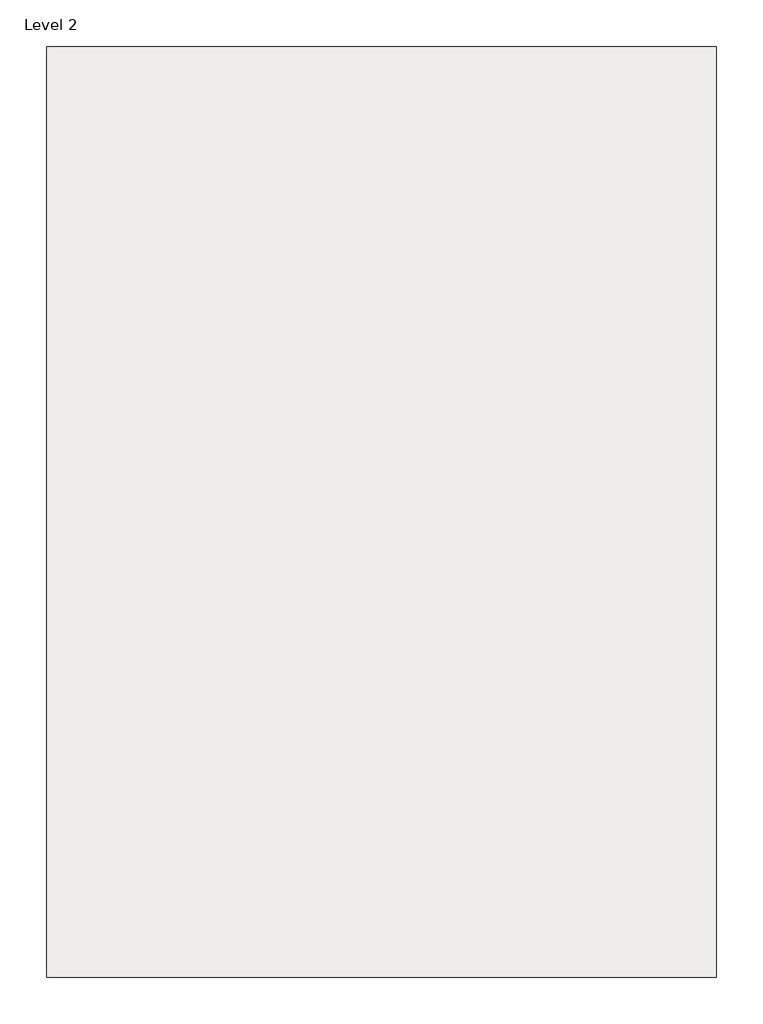
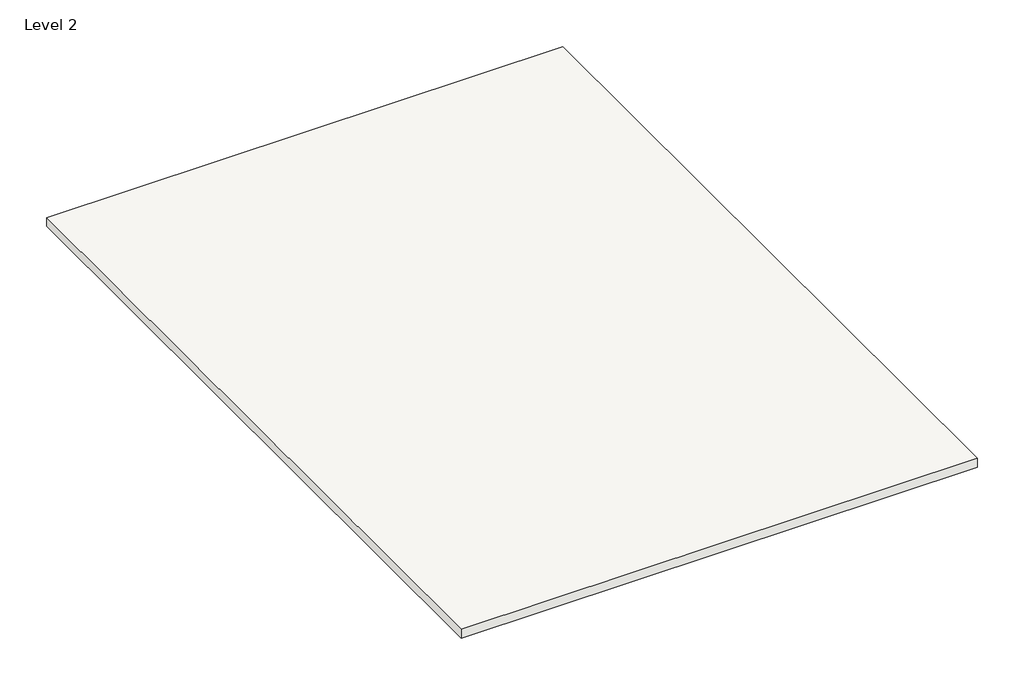
# One storey, incomplete: 1 roof.
"""IFC4 building model written with IfcOpenShell, lengths in millimetres."""

from ifc_helpers import new_model, si_unit, frame, origin, place, context, project, spatial, polyline, outline, extrude, element, save

model = new_model("IFC4")

# Units and contexts
model_context = context("Model", 3, world=origin())
ifc_project = project(units=[si_unit("LENGTHUNIT", "METRE", prefix="MILLI")], contexts=[model_context])

# Site, building, storey
site = spatial("IfcSite", under=ifc_project)
building = spatial("IfcBuilding", under=site)
storey = spatial("IfcBuildingStorey", under=building, Name="Level 2", Elevation=3048.0)

# Roof
placement = place(None, origin())
element("IfcRoof", 1, ObjectType="Generic - 12\"", at=placement, inside=storey, context=model_context, shape_type="SweptSolid", body=[
    extrude(outline(polyline([(-5216.1449167, 5769.3429147), (3115.0550833, 5769.3429147), (3115.0550833, -5813.0570853), (-5216.1449167, -5813.0570853), (-5216.1449167, 5769.3429147)])), frame((0.0, 0.0, 3048.0), z_axis=(0.0, 0.0, 1.0), x_axis=(1.0, 0.0, 0.0)), (0.0, 0.0, 1.0), 152.4),
])

save(model, "model.ifc")

# Revit data of these elements
# Type "Generic - 12\""
#   Assembly Code = "B1020"
#   Layers, outside or top first: 0' - 6" no material (function 1)
# Element 1 (IfcRoof, "Generic - 12\"")
#   built-in parameter 1001705 = 10.5 (stored number, unit not read)
#   built-in parameter 1001710 = 33615
#   Phase Created = New Construction
#   Materials on its faces: "Default Roof"
# Materials
#   "Default Roof": colour RGB 88 101 114, transparency 0, Cost = 0
